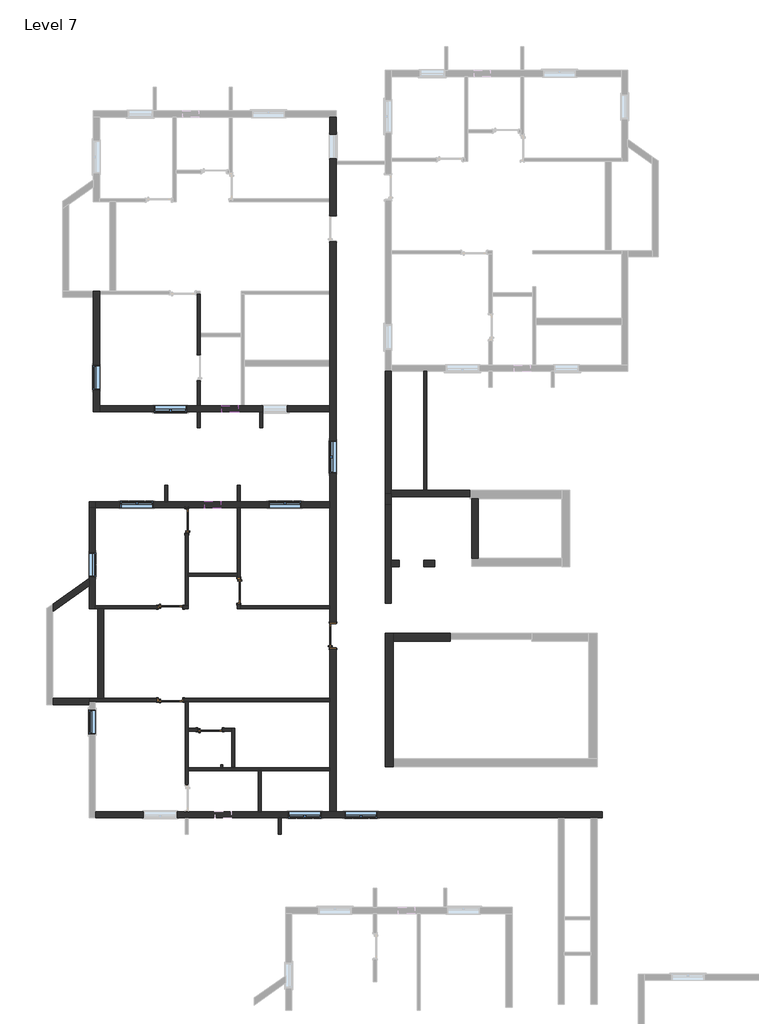
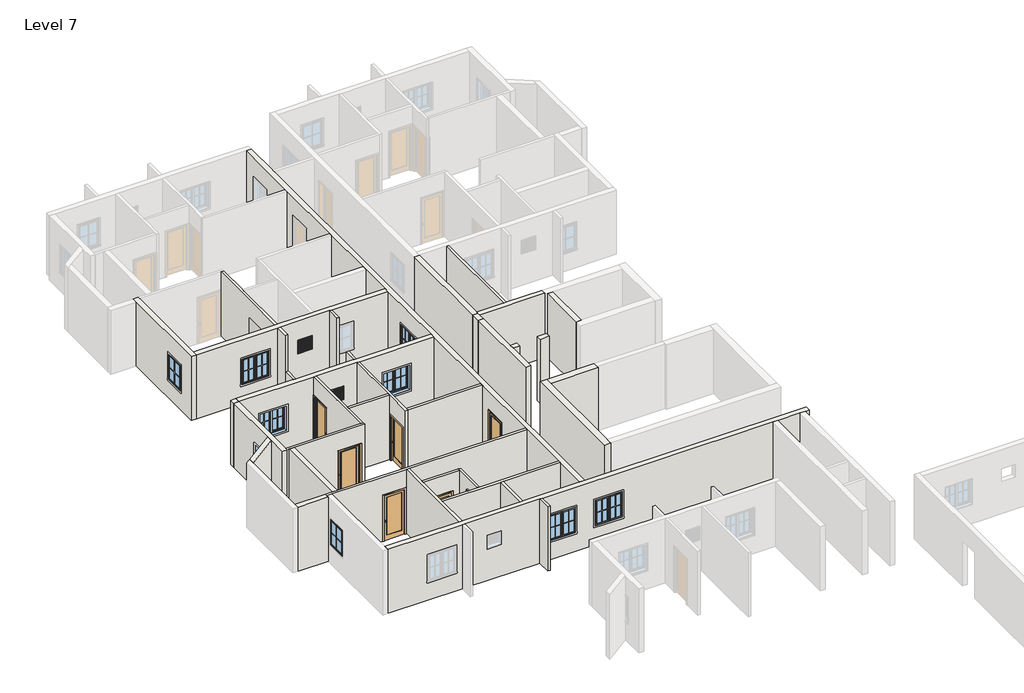
# One storey, part 4 of 7: 38 walls, 11 windows, 6 doors.
"""IFC4 building model written with IfcOpenShell, lengths in millimetres."""

from ifc_helpers import new_model, si_unit, frame, origin, place, context, project, spatial, polyline, outline, extrude, faceted_brep, transform, mapped, element, save
from components import door_a3feeac7, door_3c6ab76a, door_3b97b8e7, window_272f20d6, window_casement_double_4_x_4_af3140d2, window_f2d8fef0

model = new_model("IFC4")

# Units and contexts
model_context = context("Model", 3, world=origin())
ifc_project = project(units=[si_unit("LENGTHUNIT", "METRE", prefix="MILLI")], contexts=[model_context])

# Site, building, storey
site = spatial("IfcSite", under=ifc_project)
building = spatial("IfcBuilding", under=site)
storey = spatial("IfcBuildingStorey", under=building, Name="Level 7", Elevation=9601.2)

# Doors
placement = place(None, origin())
door_shape = door_a3feeac7(model_context)
element("IfcDoor", 1, ObjectType="Door-Interior-Single-1_Panel-Wood : 2'6\" x 7' door", at=placement, inside=storey, context=model_context, shape_type="MappedRepresentation", body=[
    mapped(door_shape, transform((-11252.4759469, 12427.2461172, 9601.2), x_axis=(0.0, 1.0, 0.0), y_axis=(-1.0, 0.0, 0.0), z_axis=(0.0, 0.0, 1.0))),
])
element("IfcDoor", 2, ObjectType="Door-Interior-Single-1_Panel-Wood : 2'6\" x 7' door", at=placement, inside=storey, context=model_context, shape_type="MappedRepresentation", body=[
    mapped(door_shape, transform((-10385.7009469, 4632.6211172, 9601.2), x_axis=(1.0, 0.0, 0.0), y_axis=(0.0, 1.0, 0.0), z_axis=(0.0, 0.0, 1.0))),
])
door_2_shape = door_3c6ab76a(model_context)
element("IfcDoor", 3, ObjectType="Door-Interior-Single-1_Panel-Wood : 36\" x 84\"", at=placement, inside=storey, context=model_context, shape_type="MappedRepresentation", body=[
    mapped(door_2_shape, transform((-9309.3759469, 9817.3961172, 9601.2), x_axis=(0.0, -1.0, 0.0), y_axis=(1.0, 0.0, 0.0), z_axis=(0.0, 0.0, 1.0))),
])
element("IfcDoor", 4, ObjectType="Door-Interior-Single-1_Panel-Wood : 36\" x 84\"", at=placement, inside=storey, context=model_context, shape_type="MappedRepresentation", body=[
    mapped(door_2_shape, transform((-11865.2509469, 9210.9711172, 9601.2), x_axis=(1.0, 0.0, 0.0), y_axis=(0.0, 1.0, 0.0), z_axis=(0.0, 0.0, 1.0))),
])
door_3_shape = door_3b97b8e7(model_context)
element("IfcDoor", 5, ObjectType="Door-Interior-Single-1_Panel-Wood : 36\" x 84\"", at=placement, inside=storey, context=model_context, shape_type="MappedRepresentation", body=[
    mapped(door_3_shape, transform((-5791.4759469, 8140.9961172, 9601.2), x_axis=(0.0, 1.0, 0.0), y_axis=(-1.0, 0.0, 0.0), z_axis=(0.0, 0.0, 1.0))),
])
element("IfcDoor", 6, ObjectType="Door-Interior-Single-1_Panel-Wood : 36\" x 84\"", at=placement, inside=storey, context=model_context, shape_type="MappedRepresentation", body=[
    mapped(door_shape, transform((-11865.2509469, 5737.5211172, 9601.2), x_axis=(1.0, 0.0, 0.0), y_axis=(0.0, 1.0, 0.0), z_axis=(0.0, 0.0, 1.0))),
])

# Walls
element("IfcWall", 7, ObjectType="1' feet", at=placement, inside=storey, context=model_context, shape_type="Brep", body=[
    faceted_brep([(-3540.4009469, 3245.1461172, 9601.2), (-3540.4009469, 3549.9461172, 9601.2), (-3540.4009469, 7931.4461172, 9601.2), (-3540.4009469, 8236.2461172, 9601.2), (-3540.4009469, 8236.2461172, 12649.2), (-3540.4009469, 7931.4461172, 12649.2), (-3540.4009469, 3549.9461172, 12649.2), (-3540.4009469, 3245.1461172, 12649.2), (-3845.2009469, 3245.1461172, 9601.2), (-3845.2009469, 3245.1461172, 12649.2), (-3845.2009469, 8236.2461172, 12649.2), (-3845.2009469, 8236.2461172, 9601.2)], [[[0, 1, 2, 3, 4, 5, 6, 7]], [[8, 9, 10, 11]], [[3, 2, 1, 0, 8, 11]], [[7, 6, 5, 4, 10, 9]], [[4, 3, 11, 10]], [[0, 7, 9, 8]]]),
])
element("IfcWall", 8, ObjectType="1' feet", at=placement, inside=storey, context=model_context, shape_type="Brep", body=[
    faceted_brep([(-3540.4009469, 7931.4461172, 9601.2), (-1406.8009469, 7931.4461172, 9601.2), (-1406.8009469, 7931.4461172, 12649.2), (-3540.4009469, 7931.4461172, 12649.2), (-3540.4009469, 8236.2461172, 9601.2), (-3540.4009469, 8236.2461172, 12649.2), (-1406.8009469, 8236.2461172, 12649.2), (-1406.8009469, 8236.2461172, 9601.2), (-1406.8009469, 8007.6461172, 9601.2), (-1406.8009469, 8007.6461172, 12649.2)], [[[0, 1, 2, 3]], [[4, 5, 6, 7]], [[1, 0, 4, 7, 8]], [[2, 1, 8, 7, 6, 9]], [[3, 2, 9, 6, 5]], [[0, 3, 5, 4]]]),
])
element("IfcWall", 9, ObjectType="4.5\" wall", at=placement, inside=storey, context=model_context, shape_type="Brep", body=[
    faceted_brep([(-10741.3009469, 20898.1461172, 12649.2), (-10741.3009469, 19437.6461172, 12649.2), (-10741.3009469, 19323.3461172, 12649.2), (-10741.3009469, 16732.5461172, 12649.2), (-10741.3009469, 16732.5461172, 9601.2), (-10741.3009469, 17678.6961172, 9601.2), (-10741.3009469, 17678.6961172, 11760.2), (-10741.3009469, 18643.8961172, 11760.2), (-10741.3009469, 18643.8961172, 9601.2), (-10741.3009469, 19323.3461172, 9601.2), (-10741.3009469, 19437.6461172, 9601.2), (-10741.3009469, 20898.1461172, 9601.2), (-10855.6009469, 16732.5461172, 12649.2), (-10855.6009469, 20898.1461172, 12649.2), (-10855.6009469, 20898.1461172, 9601.2), (-10855.6009469, 18643.8961172, 9601.2), (-10855.6009469, 18643.8961172, 11760.2), (-10855.6009469, 17678.6961172, 11760.2), (-10855.6009469, 17678.6961172, 9601.2), (-10855.6009469, 16732.5461172, 9601.2)], [[[0, 1, 2, 3, 4, 5, 6, 7, 8, 9, 10, 11]], [[12, 13, 14, 15, 16, 17, 18, 19]], [[4, 19, 18, 5]], [[14, 11, 10, 9, 8, 15]], [[3, 2, 1, 0, 13, 12]], [[4, 3, 12, 19]], [[0, 11, 14, 13]], [[7, 16, 15, 8]], [[16, 7, 6, 17]], [[17, 6, 5, 18]]]),
])
element("IfcWall", 10, ObjectType="4.5\" wall", at=placement, inside=storey, context=model_context, shape_type="Brep", body=[
    faceted_brep([(-9369.7009469, 9150.6461172, 12649.2), (-9369.7009469, 10369.8461172, 12649.2), (-9369.7009469, 10484.1461172, 12649.2), (-9369.7009469, 12922.5461172, 12649.2), (-9369.7009469, 12922.5461172, 9601.2), (-9369.7009469, 10484.1461172, 9601.2), (-9369.7009469, 10369.8461172, 9601.2), (-9369.7009469, 10299.9961172, 9601.2), (-9369.7009469, 10299.9961172, 11760.2), (-9369.7009469, 9334.7961172, 11760.2), (-9369.7009469, 9334.7961172, 9601.2), (-9369.7009469, 9150.6461172, 9601.2), (-9255.4009469, 12922.5461172, 12649.2), (-9255.4009469, 9264.9461172, 12649.2), (-9255.4009469, 9150.6461172, 12649.2), (-9255.4009469, 9150.6461172, 9601.2), (-9255.4009469, 9264.9461172, 9601.2), (-9255.4009469, 9334.7961172, 9601.2), (-9255.4009469, 9334.7961172, 11760.2), (-9255.4009469, 10299.9961172, 11760.2), (-9255.4009469, 10299.9961172, 9601.2), (-9255.4009469, 12922.5461172, 9601.2)], [[[0, 1, 2, 3, 4, 5, 6, 7, 8, 9, 10, 11]], [[12, 13, 14, 15, 16, 17, 18, 19, 20, 21]], [[4, 21, 20, 7, 6, 5]], [[15, 11, 10, 17, 16]], [[3, 2, 1, 0, 14, 13, 12]], [[4, 3, 12, 21]], [[0, 11, 15, 14]], [[9, 18, 17, 10]], [[18, 9, 8, 19]], [[19, 8, 7, 20]]]),
])
element("IfcWall", 11, ObjectType="4.5\" wall", at=placement, inside=storey, context=model_context, shape_type="SweptSolid", body=[
    extrude(outline(polyline([(-11198.5009469, 10484.1461172), (-9369.7009469, 10484.1461172), (-9369.7009469, 10369.8461172), (-11198.5009469, 10369.8461172), (-11198.5009469, 10484.1461172)])), frame((0.0, 0.0, 9601.2), z_axis=(0.0, 0.0, 1.0), x_axis=(1.0, 0.0, 0.0)), (0.0, 0.0, 1.0), 3048.0),
])
element("IfcWall", 12, ObjectType="4.5\" wall", at=placement, inside=storey, context=model_context, shape_type="Brep", body=[
    faceted_brep([(-11312.8009469, 9264.9461172, 12649.2), (-11312.8009469, 12922.5461172, 12649.2), (-11312.8009469, 12922.5461172, 9601.2), (-11312.8009469, 12909.8461172, 9601.2), (-11312.8009469, 12909.8461172, 11760.2), (-11312.8009469, 11944.6461172, 11760.2), (-11312.8009469, 11944.6461172, 9601.2), (-11312.8009469, 9264.9461172, 9601.2), (-11198.5009469, 12922.5461172, 12649.2), (-11198.5009469, 10484.1461172, 12649.2), (-11198.5009469, 10369.8461172, 12649.2), (-11198.5009469, 9264.9461172, 12649.2), (-11198.5009469, 9264.9461172, 9601.2), (-11198.5009469, 10369.8461172, 9601.2), (-11198.5009469, 10484.1461172, 9601.2), (-11198.5009469, 11944.6461172, 9601.2), (-11198.5009469, 11944.6461172, 11760.2), (-11198.5009469, 12909.8461172, 11760.2), (-11198.5009469, 12909.8461172, 9601.2), (-11198.5009469, 12922.5461172, 9601.2)], [[[0, 1, 2, 3, 4, 5, 6, 7]], [[8, 9, 10, 11, 12, 13, 14, 15, 16, 17, 18, 19]], [[12, 7, 6, 15, 14, 13]], [[2, 19, 18, 3]], [[1, 0, 11, 10, 9, 8]], [[0, 7, 12, 11]], [[2, 1, 8, 19]], [[17, 4, 3, 18]], [[4, 17, 16, 5]], [[5, 16, 15, 6]]]),
])
element("IfcWall", 13, ObjectType="4.5\" wall", at=placement, inside=storey, context=model_context, shape_type="Brep", body=[
    faceted_brep([(-14665.6009469, 9264.9461172, 12649.2), (-11312.8009469, 9264.9461172, 12649.2), (-11198.5009469, 9264.9461172, 12649.2), (-11198.5009469, 9264.9461172, 9601.2), (-11312.8009469, 9264.9461172, 9601.2), (-11382.6509469, 9264.9461172, 9601.2), (-11382.6509469, 9264.9461172, 11760.2), (-12347.8509469, 9264.9461172, 11760.2), (-12347.8509469, 9264.9461172, 9601.2), (-14665.6009469, 9264.9461172, 9601.2), (-11198.5009469, 9150.6461172, 12649.2), (-14360.8009469, 9150.6461172, 12649.2), (-14589.4009469, 9150.6461172, 12649.2), (-14665.6009469, 9150.6461172, 12649.2), (-14665.6009469, 9150.6461172, 9601.2), (-14589.4009469, 9150.6461172, 9601.2), (-14360.8009469, 9150.6461172, 9601.2), (-12347.8509469, 9150.6461172, 9601.2), (-12347.8509469, 9150.6461172, 11760.2), (-11382.6509469, 9150.6461172, 11760.2), (-11382.6509469, 9150.6461172, 9601.2), (-11198.5009469, 9150.6461172, 9601.2)], [[[0, 1, 2, 3, 4, 5, 6, 7, 8, 9]], [[10, 11, 12, 13, 14, 15, 16, 17, 18, 19, 20, 21]], [[3, 21, 20, 5, 4]], [[14, 9, 8, 17, 16, 15]], [[2, 1, 0, 13, 12, 11, 10]], [[3, 2, 10, 21]], [[0, 9, 14, 13]], [[19, 6, 5, 20]], [[6, 19, 18, 7]], [[7, 18, 17, 8]]]),
])
element("IfcWall", 14, ObjectType="4.5\" wall", at=placement, inside=storey, context=model_context, shape_type="SweptSolid", body=[
    extrude(outline(polyline([(-9255.4009469, 9264.9461172), (-5902.6009469, 9264.9461172), (-5902.6009469, 9150.6461172), (-9255.4009469, 9150.6461172), (-9255.4009469, 9264.9461172)])), frame((0.0, 0.0, 9601.2), z_axis=(0.0, 0.0, 1.0), x_axis=(1.0, 0.0, 0.0)), (0.0, 0.0, 1.0), 3048.0),
])
element("IfcWall", 15, ObjectType="4.5\" wall", at=placement, inside=storey, context=model_context, shape_type="Brep", body=[
    faceted_brep([(-5902.6009469, 5683.5461172, 12649.2), (-11198.5009469, 5683.5461172, 12649.2), (-11312.8009469, 5683.5461172, 12649.2), (-14665.6009469, 5683.5461172, 12649.2), (-14894.2009469, 5683.5461172, 12649.2), (-14894.2009469, 5683.5461172, 9601.2), (-14665.6009469, 5683.5461172, 9601.2), (-12347.8509469, 5683.5461172, 9601.2), (-12347.8509469, 5683.5461172, 11760.2), (-11382.6509469, 5683.5461172, 11760.2), (-11382.6509469, 5683.5461172, 9601.2), (-11312.8009469, 5683.5461172, 9601.2), (-11198.5009469, 5683.5461172, 9601.2), (-5902.6009469, 5683.5461172, 9601.2), (-14894.2009469, 5797.8461172, 12649.2), (-14589.4009469, 5797.8461172, 12649.2), (-14360.8009469, 5797.8461172, 12649.2), (-5902.6009469, 5797.8461172, 12649.2), (-5902.6009469, 5797.8461172, 9601.2), (-11382.6509469, 5797.8461172, 9601.2), (-11382.6509469, 5797.8461172, 11760.2), (-12347.8509469, 5797.8461172, 11760.2), (-12347.8509469, 5797.8461172, 9601.2), (-14360.8009469, 5797.8461172, 9601.2), (-14589.4009469, 5797.8461172, 9601.2), (-14894.2009469, 5797.8461172, 9601.2)], [[[0, 1, 2, 3, 4, 5, 6, 7, 8, 9, 10, 11, 12, 13]], [[14, 15, 16, 17, 18, 19, 20, 21, 22, 23, 24, 25]], [[18, 13, 12, 11, 10, 19]], [[5, 25, 24, 23, 22, 7, 6]], [[4, 3, 2, 1, 0, 17, 16, 15, 14]], [[0, 13, 18, 17]], [[5, 4, 14, 25]], [[9, 20, 19, 10]], [[20, 9, 8, 21]], [[21, 8, 7, 22]]]),
])
element("IfcWall", 16, ObjectType="4.5\" wall", at=placement, inside=storey, context=model_context, shape_type="Brep", body=[
    faceted_brep([(-11198.5009469, 5683.5461172, 12649.2), (-11198.5009469, 4692.9461172, 12649.2), (-11198.5009469, 4578.6461172, 12649.2), (-11198.5009469, 3207.0461172, 12649.2), (-11198.5009469, 3092.7461172, 12649.2), (-11198.5009469, 1568.7461172, 12649.2), (-11198.5009469, 1568.7461172, 9601.2), (-11198.5009469, 1581.4461172, 9601.2), (-11198.5009469, 1581.4461172, 11760.2), (-11198.5009469, 2546.6461172, 11760.2), (-11198.5009469, 2546.6461172, 9601.2), (-11198.5009469, 3092.7461172, 9601.2), (-11198.5009469, 3207.0461172, 9601.2), (-11198.5009469, 4578.6461172, 9601.2), (-11198.5009469, 4692.9461172, 9601.2), (-11198.5009469, 5683.5461172, 9601.2), (-11312.8009469, 1568.7461172, 12649.2), (-11312.8009469, 5683.5461172, 12649.2), (-11312.8009469, 5683.5461172, 9601.2), (-11312.8009469, 2546.6461172, 9601.2), (-11312.8009469, 2546.6461172, 11760.2), (-11312.8009469, 1581.4461172, 11760.2), (-11312.8009469, 1581.4461172, 9601.2), (-11312.8009469, 1568.7461172, 9601.2)], [[[0, 1, 2, 3, 4, 5, 6, 7, 8, 9, 10, 11, 12, 13, 14, 15]], [[16, 17, 18, 19, 20, 21, 22, 23]], [[18, 15, 14, 13, 12, 11, 10, 19]], [[6, 23, 22, 7]], [[5, 4, 3, 2, 1, 0, 17, 16]], [[0, 15, 18, 17]], [[6, 5, 16, 23]], [[21, 8, 7, 22]], [[8, 21, 20, 9]], [[9, 20, 19, 10]]]),
])
element("IfcWall", 17, ObjectType="4.5\" wall", at=placement, inside=storey, context=model_context, shape_type="SweptSolid", body=[
    extrude(outline(polyline([(-9985.226836, 3326.5226372), (-9915.376836, 3326.5226372), (-9915.376836, 3212.2226372), (-9985.226836, 3212.2226372), (-9985.226836, 3326.5226372)])), frame((0.0, 0.0, 9601.2), z_axis=(0.0, 0.0, 1.0), x_axis=(1.0, 0.0, 0.0)), (0.0, 0.0, 1.0), 3048.0),
])
element("IfcWall", 18, ObjectType="4.5\" wall", at=placement, inside=storey, context=model_context, shape_type="Brep", body=[
    faceted_brep([(-5902.6009469, 3207.0461172, 9601.2), (-11198.5009469, 3207.0461172, 9601.2), (-11198.5009469, 3207.0461172, 12649.2), (-5902.6009469, 3207.0461172, 12649.2), (-5902.6009469, 3092.7461172, 9601.2), (-5902.6009469, 3092.7461172, 12649.2), (-8468.0009469, 3092.7461172, 12649.2), (-8582.3009469, 3092.7461172, 12649.2), (-11198.5009469, 3092.7461172, 12649.2), (-11198.5009469, 3092.7461172, 9601.2), (-8582.3009469, 3092.7461172, 9601.2), (-8468.0009469, 3092.7461172, 9601.2)], [[[0, 1, 2, 3]], [[4, 5, 6, 7, 8, 9, 10, 11]], [[1, 0, 4, 11, 10, 9]], [[3, 2, 8, 7, 6, 5]], [[2, 1, 9, 8]], [[0, 3, 5, 4]]]),
])
element("IfcWall", 19, ObjectType="4.5\" wall", at=placement, inside=storey, context=model_context, shape_type="SweptSolid", body=[
    extrude(outline(polyline([(-8582.3009469, 1568.7461172), (-8582.3009469, 3092.7461172), (-8468.0009469, 3092.7461172), (-8468.0009469, 1568.7461172), (-8582.3009469, 1568.7461172)])), frame((0.0, 0.0, 9601.2), z_axis=(0.0, 0.0, 1.0), x_axis=(1.0, 0.0, 0.0)), (0.0, 0.0, 1.0), 3048.0),
])
element("IfcWall", 20, ObjectType="4.5\" wall", at=placement, inside=storey, context=model_context, shape_type="Brep", body=[
    faceted_brep([(-9572.9009469, 4692.9461172, 9601.2), (-9572.9009469, 4578.6461172, 9601.2), (-9572.9009469, 3245.1461172, 9601.2), (-9572.9009469, 3245.1461172, 12649.2), (-9572.9009469, 4578.6461172, 12649.2), (-9572.9009469, 4692.9461172, 12649.2), (-9458.6009469, 4692.9461172, 9601.2), (-9458.6009469, 4692.9461172, 12649.2), (-9458.6009469, 3245.1461172, 12649.2), (-9458.6009469, 3245.1461172, 9601.2)], [[[0, 1, 2, 3, 4, 5]], [[6, 7, 8, 9]], [[2, 1, 0, 6, 9]], [[3, 2, 9, 8]], [[5, 4, 3, 8, 7]], [[0, 5, 7, 6]]]),
])
element("IfcWall", 21, ObjectType="4.5\" wall", at=placement, inside=storey, context=model_context, shape_type="SweptSolid", body=[
    extrude(outline(polyline([(12649.2, -9572.9009469), (12649.2, -11198.5009469), (9601.2, -11198.5009469), (9601.2, -10868.3009469), (11760.2, -10868.3009469), (11760.2, -9903.1009469), (9601.2, -9903.1009469), (9601.2, -9572.9009469), (12649.2, -9572.9009469)])), frame((0.0, 4578.6461172, 0.0), z_axis=(0.0, 1.0, 0.0), x_axis=(0.0, 0.0, 1.0)), (0.0, 0.0, 1.0), 114.3),
])
element("IfcWall", 22, ObjectType="4.5\" wall", at=placement, inside=storey, context=model_context, shape_type="SweptSolid", body=[
    extrude(outline(polyline([(-7841.0333092, 730.5461172), (-7841.0333092, 1340.1461172), (-7726.7333092, 1340.1461172), (-7726.7333092, 730.5461172), (-7841.0333092, 730.5461172)])), frame((0.0, 0.0, 9601.2), z_axis=(0.0, 0.0, 1.0), x_axis=(1.0, 0.0, 0.0)), (0.0, 0.0, 1.0), 3048.0),
])
element("IfcWall", 23, ObjectType="4.5\" wall", at=placement, inside=storey, context=model_context, shape_type="SweptSolid", body=[
    extrude(outline(polyline([(-10855.6009469, 15918.3895495), (-10855.6009469, 16503.9461172), (-10741.3009469, 16503.9461172), (-10741.3009469, 15918.3895495), (-10855.6009469, 15918.3895495)])), frame((0.0, 0.0, 9601.2), z_axis=(0.0, 0.0, 1.0), x_axis=(1.0, 0.0, 0.0)), (0.0, 0.0, 1.0), 3048.0),
])
element("IfcWall", 24, ObjectType="4.5\" wall", at=placement, inside=storey, context=model_context, shape_type="Brep", body=[
    faceted_brep([(-8531.5009469, 16503.9461172, 9601.2), (-8531.5009469, 15918.3895495, 9601.2), (-8531.5009469, 15918.3895495, 12649.2), (-8531.5009469, 16503.9461172, 12649.2), (-8417.2009469, 16503.9461172, 9601.2), (-8417.2009469, 16503.9461172, 10515.6), (-8417.2009469, 16503.9461172, 11734.8), (-8417.2009469, 16503.9461172, 12649.2), (-8417.2009469, 15918.3895495, 12649.2), (-8417.2009469, 15918.3895495, 9601.2)], [[[0, 1, 2, 3]], [[4, 5, 6, 7, 8, 9]], [[1, 0, 4, 9]], [[2, 1, 9, 8]], [[3, 2, 8, 7]], [[0, 3, 7, 6, 5, 4]]]),
])
element("IfcWall", 25, ObjectType="4.5\" wall", at=placement, inside=storey, context=model_context, shape_type="SweptSolid", body=[
    extrude(outline(polyline([(-12085.9698258, 13151.1461172), (-12085.9698258, 13760.7461172), (-11971.6698258, 13760.7461172), (-11971.6698258, 13151.1461172), (-12085.9698258, 13151.1461172)])), frame((0.0, 0.0, 9601.2), z_axis=(0.0, 0.0, 1.0), x_axis=(1.0, 0.0, 0.0)), (0.0, 0.0, 1.0), 3048.0),
])
element("IfcWall", 26, ObjectType="4.5\" wall", at=placement, inside=storey, context=model_context, shape_type="SweptSolid", body=[
    extrude(outline(polyline([(-9255.4009469, 13760.7461172), (-9255.4009469, 13151.1461172), (-9369.7009469, 13151.1461172), (-9369.7009469, 13760.7461172), (-9255.4009469, 13760.7461172)])), frame((0.0, 0.0, 9601.2), z_axis=(0.0, 0.0, 1.0), x_axis=(1.0, 0.0, 0.0)), (0.0, 0.0, 1.0), 3048.0),
])
element("IfcWall", 27, ObjectType="4.5\" wall", at=placement, inside=storey, context=model_context, shape_type="SweptSolid", body=[
    extrude(outline(polyline([(-2402.381873, 13571.4182723), (-2402.381873, 18017.4255084), (-2288.081873, 18017.4255084), (-2288.081873, 13571.4182723), (-2402.381873, 13571.4182723)])), frame((0.0, 0.0, 9601.2), z_axis=(0.0, 0.0, 1.0), x_axis=(1.0, 0.0, 0.0)), (0.0, 0.0, 1.0), 3048.0),
])
element("IfcWall", 28, ObjectType="9\"", at=placement, inside=storey, context=model_context, shape_type="Brep", body=[
    faceted_brep([(-14513.2009469, 16503.9461172, 9601.2), (-14513.2009469, 16732.5461172, 9601.2), (-14513.2009469, 20898.1461172, 9601.2), (-14513.2009469, 21012.4461172, 9601.2), (-14513.2009469, 21012.4461172, 12649.2), (-14513.2009469, 20898.1461172, 12649.2), (-14513.2009469, 16732.5461172, 12649.2), (-14513.2009469, 16503.9461172, 12649.2), (-14513.2009469, 18243.8461172, 11734.8), (-14513.2009469, 18243.8461172, 10515.6), (-14513.2009469, 17329.4461172, 10515.6), (-14513.2009469, 17329.4461172, 11734.8), (-14741.8009469, 16503.9461172, 9601.2), (-14741.8009469, 16503.9461172, 12649.2), (-14741.8009469, 20783.8461172, 12649.2), (-14741.8009469, 21012.4461172, 12649.2), (-14741.8009469, 21012.4461172, 9601.2), (-14741.8009469, 20783.8461172, 9601.2), (-14741.8009469, 18243.8461172, 11734.8), (-14741.8009469, 17329.4461172, 11734.8), (-14741.8009469, 17329.4461172, 10515.6), (-14741.8009469, 18243.8461172, 10515.6)], [[[0, 1, 2, 3, 4, 5, 6, 7], [8, 9, 10, 11]], [[12, 13, 14, 15, 16, 17], [18, 19, 20, 21]], [[3, 2, 1, 0, 12, 17, 16]], [[7, 6, 5, 4, 15, 14, 13]], [[4, 3, 16, 15]], [[0, 7, 13, 12]], [[9, 8, 18, 21]], [[10, 9, 21, 20]], [[11, 10, 20, 19]], [[8, 11, 19, 18]]]),
])
element("IfcWall", 29, ObjectType="9\"", at=placement, inside=storey, context=model_context, shape_type="Brep", body=[
    faceted_brep([(-5902.6009469, 1568.7461172, 12649.2), (-5902.6009469, 3092.7461172, 12649.2), (-5902.6009469, 3207.0461172, 12649.2), (-5902.6009469, 5683.5461172, 12649.2), (-5902.6009469, 5797.8461172, 12649.2), (-5902.6009469, 9150.6461172, 12649.2), (-5902.6009469, 9264.9461172, 12649.2), (-5902.6009469, 12922.5461172, 12649.2), (-5902.6009469, 13151.1461172, 12649.2), (-5902.6009469, 16503.9461172, 12649.2), (-5902.6009469, 16732.5461172, 12649.2), (-5902.6009469, 18205.7461172, 12649.2), (-5902.6009469, 18434.3461172, 12649.2), (-5902.6009469, 20898.1461172, 12649.2), (-5902.6009469, 21012.4461172, 12649.2), (-5902.6009469, 24365.2461172, 12649.2), (-5902.6009469, 24479.5461172, 12649.2), (-5902.6009469, 27527.5461172, 12649.2), (-5902.6009469, 27527.5461172, 9601.2), (-5902.6009469, 24479.5461172, 9601.2), (-5902.6009469, 24365.2461172, 9601.2), (-5902.6009469, 23838.1961172, 9601.2), (-5902.6009469, 23838.1961172, 11760.2), (-5902.6009469, 22872.9961172, 11760.2), (-5902.6009469, 22872.9961172, 9601.2), (-5902.6009469, 21012.4461172, 9601.2), (-5902.6009469, 20898.1461172, 9601.2), (-5902.6009469, 18434.3461172, 9601.2), (-5902.6009469, 18205.7461172, 9601.2), (-5902.6009469, 16732.5461172, 9601.2), (-5902.6009469, 16503.9461172, 9601.2), (-5902.6009469, 13151.1461172, 9601.2), (-5902.6009469, 12922.5461172, 9601.2), (-5902.6009469, 9264.9461172, 9601.2), (-5902.6009469, 9150.6461172, 9601.2), (-5902.6009469, 8623.5961172, 9601.2), (-5902.6009469, 8623.5961172, 11760.2), (-5902.6009469, 7658.3961172, 11760.2), (-5902.6009469, 7658.3961172, 9601.2), (-5902.6009469, 5797.8461172, 9601.2), (-5902.6009469, 5683.5461172, 9601.2), (-5902.6009469, 3207.0461172, 9601.2), (-5902.6009469, 3092.7461172, 9601.2), (-5902.6009469, 1568.7461172, 9601.2), (-5902.6009469, 25973.9755084, 11734.8), (-5902.6009469, 25973.9755084, 10515.6), (-5902.6009469, 26888.3755084, 10515.6), (-5902.6009469, 26888.3755084, 11734.8), (-5902.6009469, 15437.1461172, 11734.8), (-5902.6009469, 14217.9461172, 11734.8), (-5902.6009469, 14217.9461172, 10515.6), (-5902.6009469, 15437.1461172, 10515.6), (-5674.0009469, 27527.5461172, 12649.2), (-5674.0009469, 25878.7255084, 12649.2), (-5674.0009469, 25764.4255084, 12649.2), (-5674.0009469, 1568.7461172, 12649.2), (-5674.0009469, 1568.7461172, 9601.2), (-5674.0009469, 7658.3961172, 9601.2), (-5674.0009469, 7658.3961172, 11760.2), (-5674.0009469, 8623.5961172, 11760.2), (-5674.0009469, 8623.5961172, 9601.2), (-5674.0009469, 22872.9961172, 9601.2), (-5674.0009469, 22872.9961172, 11760.2), (-5674.0009469, 23838.1961172, 11760.2), (-5674.0009469, 23838.1961172, 9601.2), (-5674.0009469, 25764.4255084, 9601.2), (-5674.0009469, 25878.7255084, 9601.2), (-5674.0009469, 27527.5461172, 9601.2), (-5674.0009469, 27527.5461172, 9753.6), (-5674.0009469, 25973.9755084, 11734.8), (-5674.0009469, 26888.3755084, 11734.8), (-5674.0009469, 26888.3755084, 10515.6), (-5674.0009469, 25973.9755084, 10515.6), (-5674.0009469, 15437.1461172, 11734.8), (-5674.0009469, 15437.1461172, 10515.6), (-5674.0009469, 14217.9461172, 10515.6), (-5674.0009469, 14217.9461172, 11734.8)], [[[0, 1, 2, 3, 4, 5, 6, 7, 8, 9, 10, 11, 12, 13, 14, 15, 16, 17, 18, 19, 20, 21, 22, 23, 24, 25, 26, 27, 28, 29, 30, 31, 32, 33, 34, 35, 36, 37, 38, 39, 40, 41, 42, 43], [44, 45, 46, 47], [48, 49, 50, 51]], [[52, 53, 54, 55, 56, 57, 58, 59, 60, 61, 62, 63, 64, 65, 66, 67, 68], [69, 70, 71, 72], [73, 74, 75, 76]], [[18, 67, 66, 65, 64, 21, 20, 19]], [[56, 43, 42, 41, 40, 39, 38, 57]], [[24, 61, 60, 35, 34, 33, 32, 31, 30, 29, 28, 27, 26, 25]], [[17, 16, 15, 14, 13, 12, 11, 10, 9, 8, 7, 6, 5, 4, 3, 2, 1, 0, 55, 54, 53, 52]], [[18, 17, 52, 68, 67]], [[0, 43, 56, 55]], [[63, 22, 21, 64]], [[22, 63, 62, 23]], [[23, 62, 61, 24]], [[59, 36, 35, 60]], [[36, 59, 58, 37]], [[37, 58, 57, 38]], [[45, 44, 69, 72]], [[46, 45, 72, 71]], [[47, 46, 71, 70]], [[44, 47, 70, 69]], [[74, 73, 48, 51]], [[75, 74, 51, 50]], [[76, 75, 50, 49]], [[73, 76, 49, 48]]]),
])
element("IfcWall", 30, ObjectType="9\"", at=placement, inside=storey, context=model_context, shape_type="Brep", body=[
    faceted_brep([(-14513.2009469, 16503.9461172, 9601.2), (-10855.6009469, 16503.9461172, 9601.2), (-10741.3009469, 16503.9461172, 9601.2), (-8531.5009469, 16503.9461172, 9601.2), (-8417.2009469, 16503.9461172, 9601.2), (-5902.6009469, 16503.9461172, 9601.2), (-5902.6009469, 16503.9461172, 12649.2), (-8417.2009469, 16503.9461172, 12649.2), (-8531.5009469, 16503.9461172, 12649.2), (-10741.3009469, 16503.9461172, 12649.2), (-10855.6009469, 16503.9461172, 12649.2), (-14513.2009469, 16503.9461172, 12649.2), (-9337.9509469, 16503.9461172, 11734.8), (-9337.9509469, 16503.9461172, 11125.2), (-9947.5509469, 16503.9461172, 11125.2), (-9947.5509469, 16503.9461172, 11734.8), (-8417.2009469, 16503.9461172, 11734.8), (-7502.8009469, 16503.9461172, 11734.8), (-7502.8009469, 16503.9461172, 10515.6), (-8417.2009469, 16503.9461172, 10515.6), (-12474.8509469, 16503.9461172, 11734.8), (-11255.6509469, 16503.9461172, 11734.8), (-11255.6509469, 16503.9461172, 10515.6), (-12474.8509469, 16503.9461172, 10515.6), (-14513.2009469, 16732.5461172, 9601.2), (-14513.2009469, 16732.5461172, 12649.2), (-10855.6009469, 16732.5461172, 12649.2), (-10741.3009469, 16732.5461172, 12649.2), (-9217.3009469, 16732.5461172, 12649.2), (-9103.0009469, 16732.5461172, 12649.2), (-5902.6009469, 16732.5461172, 12649.2), (-5902.6009469, 16732.5461172, 9601.2), (-9103.0009469, 16732.5461172, 9601.2), (-9217.3009469, 16732.5461172, 9601.2), (-10741.3009469, 16732.5461172, 9601.2), (-10855.6009469, 16732.5461172, 9601.2), (-9337.9509469, 16732.5461172, 11734.8), (-9947.5509469, 16732.5461172, 11734.8), (-9947.5509469, 16732.5461172, 11125.2), (-9337.9509469, 16732.5461172, 11125.2), (-8417.2009469, 16732.5461172, 11734.8), (-8417.2009469, 16732.5461172, 10515.6), (-7502.8009469, 16732.5461172, 10515.6), (-7502.8009469, 16732.5461172, 11734.8), (-12474.8509469, 16732.5461172, 11734.8), (-12474.8509469, 16732.5461172, 10515.6), (-11255.6509469, 16732.5461172, 10515.6), (-11255.6509469, 16732.5461172, 11734.8)], [[[0, 1, 2, 3, 4, 5, 6, 7, 8, 9, 10, 11], [12, 13, 14, 15], [16, 17, 18, 19], [20, 21, 22, 23]], [[24, 25, 26, 27, 28, 29, 30, 31, 32, 33, 34, 35], [36, 37, 38, 39], [40, 41, 42, 43], [44, 45, 46, 47]], [[5, 4, 3, 2, 1, 0, 24, 35, 34, 33, 32, 31]], [[11, 10, 9, 8, 7, 6, 30, 29, 28, 27, 26, 25]], [[6, 5, 31, 30]], [[0, 11, 25, 24]], [[13, 12, 36, 39]], [[14, 13, 39, 38]], [[15, 14, 38, 37]], [[12, 15, 37, 36]], [[41, 40, 16, 19]], [[42, 41, 19, 18]], [[43, 42, 18, 17]], [[40, 43, 17, 16]], [[45, 44, 20, 23]], [[46, 45, 23, 22]], [[47, 46, 22, 21]], [[44, 47, 21, 20]]]),
])
element("IfcWall", 31, ObjectType="9\"", at=placement, inside=storey, context=model_context, shape_type="Brep", body=[
    faceted_brep([(-5902.6009469, 13151.1461172, 9601.2), (-9255.4009469, 13151.1461172, 9601.2), (-9369.7009469, 13151.1461172, 9601.2), (-11971.6698258, 13151.1461172, 9601.2), (-12085.9698258, 13151.1461172, 9601.2), (-14665.6009469, 13151.1461172, 9601.2), (-14665.6009469, 13151.1461172, 12649.2), (-12085.9698258, 13151.1461172, 12649.2), (-11971.6698258, 13151.1461172, 12649.2), (-9369.7009469, 13151.1461172, 12649.2), (-9255.4009469, 13151.1461172, 12649.2), (-5902.6009469, 13151.1461172, 12649.2), (-9979.3009469, 13151.1461172, 11734.8), (-10588.9009469, 13151.1461172, 11734.8), (-10588.9009469, 13151.1461172, 11125.2), (-9979.3009469, 13151.1461172, 11125.2), (-12511.4198258, 13151.1461172, 11734.8), (-13730.6198258, 13151.1461172, 11734.8), (-13730.6198258, 13151.1461172, 10515.6), (-12511.4198258, 13151.1461172, 10515.6), (-6975.7509469, 13151.1461172, 11734.8), (-8194.9509469, 13151.1461172, 11734.8), (-8194.9509469, 13151.1461172, 10515.6), (-6975.7509469, 13151.1461172, 10515.6), (-5902.6009469, 12922.5461172, 9601.2), (-5902.6009469, 12922.5461172, 12649.2), (-9255.4009469, 12922.5461172, 12649.2), (-9369.7009469, 12922.5461172, 12649.2), (-11198.5009469, 12922.5461172, 12649.2), (-11312.8009469, 12922.5461172, 12649.2), (-14665.6009469, 12922.5461172, 12649.2), (-14665.6009469, 12922.5461172, 9601.2), (-11312.8009469, 12922.5461172, 9601.2), (-11198.5009469, 12922.5461172, 9601.2), (-9369.7009469, 12922.5461172, 9601.2), (-9255.4009469, 12922.5461172, 9601.2), (-9979.3009469, 12922.5461172, 11734.8), (-9979.3009469, 12922.5461172, 11125.2), (-10588.9009469, 12922.5461172, 11125.2), (-10588.9009469, 12922.5461172, 11734.8), (-12511.4198258, 12922.5461172, 11734.8), (-12511.4198258, 12922.5461172, 10515.6), (-13730.6198258, 12922.5461172, 10515.6), (-13730.6198258, 12922.5461172, 11734.8), (-6975.7509469, 12922.5461172, 11734.8), (-6975.7509469, 12922.5461172, 10515.6), (-8194.9509469, 12922.5461172, 10515.6), (-8194.9509469, 12922.5461172, 11734.8)], [[[0, 1, 2, 3, 4, 5, 6, 7, 8, 9, 10, 11], [12, 13, 14, 15], [16, 17, 18, 19], [20, 21, 22, 23]], [[24, 25, 26, 27, 28, 29, 30, 31, 32, 33, 34, 35], [36, 37, 38, 39], [40, 41, 42, 43], [44, 45, 46, 47]], [[5, 4, 3, 2, 1, 0, 24, 35, 34, 33, 32, 31]], [[11, 10, 9, 8, 7, 6, 30, 29, 28, 27, 26, 25]], [[6, 5, 31, 30]], [[0, 11, 25, 24]], [[37, 36, 12, 15]], [[38, 37, 15, 14]], [[39, 38, 14, 13]], [[36, 39, 13, 12]], [[41, 40, 16, 19]], [[42, 41, 19, 18]], [[43, 42, 18, 17]], [[40, 43, 17, 16]], [[45, 44, 20, 23]], [[46, 45, 23, 22]], [[47, 46, 22, 21]], [[44, 47, 21, 20]]]),
])
element("IfcWall", 32, ObjectType="9\"", at=placement, inside=storey, context=model_context, shape_type="SweptSolid", body=[
    extrude(outline(polyline([(-14894.2009469, 12922.5461172), (-14894.2009469, 13151.1461172), (-14665.6009469, 13151.1461172), (-14665.6009469, 12922.5461172), (-14894.2009469, 12922.5461172)])), frame((0.0, 0.0, 9601.2), z_axis=(0.0, 0.0, 1.0), x_axis=(1.0, 0.0, 0.0)), (0.0, 0.0, 1.0), 3048.0),
])
element("IfcWall", 33, ObjectType="9\"", at=placement, inside=storey, context=model_context, shape_type="SweptSolid", body=[
    extrude(outline(polyline([(-14589.4009469, 5797.8461172), (-14589.4009469, 9150.6461172), (-14360.8009469, 9150.6461172), (-14360.8009469, 5797.8461172), (-14589.4009469, 5797.8461172)])), frame((0.0, 0.0, 9601.2), z_axis=(0.0, 0.0, 1.0), x_axis=(1.0, 0.0, 0.0)), (0.0, 0.0, 1.0), 3048.0),
])
element("IfcWall", 34, ObjectType="9\"", at=placement, inside=storey, context=model_context, shape_type="Brep", body=[
    faceted_brep([(-14665.6009469, 1340.1461172, 9601.2), (-11312.8009469, 1340.1461172, 9601.2), (-11198.5009469, 1340.1461172, 9601.2), (-7841.0333092, 1340.1461172, 9601.2), (-7726.7333092, 1340.1461172, 9601.2), (2631.7990531, 1340.1461172, 9601.2), (2860.3990531, 1340.1461172, 9601.2), (3850.9990531, 1340.1461172, 9601.2), (4079.5990531, 1340.1461172, 9601.2), (4270.0990531, 1340.1461172, 9601.2), (4270.0990531, 1340.1461172, 12649.2), (4079.5990531, 1340.1461172, 12649.2), (3850.9990531, 1340.1461172, 12649.2), (2860.3990531, 1340.1461172, 12649.2), (2631.7990531, 1340.1461172, 12649.2), (-7726.7333092, 1340.1461172, 12649.2), (-7841.0333092, 1340.1461172, 12649.2), (-11198.5009469, 1340.1461172, 12649.2), (-11312.8009469, 1340.1461172, 12649.2), (-14665.6009469, 1340.1461172, 12649.2), (-10195.2009469, 1340.1461172, 11734.8), (-9585.6009469, 1340.1461172, 11734.8), (-9585.6009469, 1340.1461172, 11125.2), (-10195.2009469, 1340.1461172, 11125.2), (-5356.5009469, 1340.1461172, 11734.8), (-4137.3009469, 1340.1461172, 11734.8), (-4137.3009469, 1340.1461172, 10515.6), (-5356.5009469, 1340.1461172, 10515.6), (-7453.6833092, 1340.1461172, 11734.8), (-6234.4833092, 1340.1461172, 11734.8), (-6234.4833092, 1340.1461172, 10515.6), (-7453.6833092, 1340.1461172, 10515.6), (-12855.8509469, 1340.1461172, 11734.8), (-11636.6509469, 1340.1461172, 11734.8), (-11636.6509469, 1340.1461172, 10515.6), (-12855.8509469, 1340.1461172, 10515.6), (-14665.6009469, 1568.7461172, 9601.2), (-14665.6009469, 1568.7461172, 12649.2), (-11312.8009469, 1568.7461172, 12649.2), (-11198.5009469, 1568.7461172, 12649.2), (-8582.3009469, 1568.7461172, 12649.2), (-8468.0009469, 1568.7461172, 12649.2), (-5902.6009469, 1568.7461172, 12649.2), (-5674.0009469, 1568.7461172, 12649.2), (4270.0990531, 1568.7461172, 12649.2), (4270.0990531, 1568.7461172, 9601.2), (-5674.0009469, 1568.7461172, 9601.2), (-5902.6009469, 1568.7461172, 9601.2), (-8468.0009469, 1568.7461172, 9601.2), (-8582.3009469, 1568.7461172, 9601.2), (-11198.5009469, 1568.7461172, 9601.2), (-11312.8009469, 1568.7461172, 9601.2), (-10195.2009469, 1568.7461172, 11734.8), (-10195.2009469, 1568.7461172, 11125.2), (-9585.6009469, 1568.7461172, 11125.2), (-9585.6009469, 1568.7461172, 11734.8), (-5356.5009469, 1568.7461172, 11734.8), (-5356.5009469, 1568.7461172, 10515.6), (-4137.3009469, 1568.7461172, 10515.6), (-4137.3009469, 1568.7461172, 11734.8), (-7453.6833092, 1568.7461172, 11734.8), (-7453.6833092, 1568.7461172, 10515.6), (-6234.4833092, 1568.7461172, 10515.6), (-6234.4833092, 1568.7461172, 11734.8), (-12855.8509469, 1568.7461172, 11734.8), (-12855.8509469, 1568.7461172, 10515.6), (-11636.6509469, 1568.7461172, 10515.6), (-11636.6509469, 1568.7461172, 11734.8)], [[[0, 1, 2, 3, 4, 5, 6, 7, 8, 9, 10, 11, 12, 13, 14, 15, 16, 17, 18, 19], [20, 21, 22, 23], [24, 25, 26, 27], [28, 29, 30, 31], [32, 33, 34, 35]], [[36, 37, 38, 39, 40, 41, 42, 43, 44, 45, 46, 47, 48, 49, 50, 51], [52, 53, 54, 55], [56, 57, 58, 59], [60, 61, 62, 63], [64, 65, 66, 67]], [[9, 8, 7, 6, 5, 4, 3, 2, 1, 0, 36, 51, 50, 49, 48, 47, 46, 45]], [[10, 9, 45, 44]], [[19, 18, 17, 16, 15, 14, 13, 12, 11, 10, 44, 43, 42, 41, 40, 39, 38, 37]], [[0, 19, 37, 36]], [[53, 52, 20, 23]], [[54, 53, 23, 22]], [[55, 54, 22, 21]], [[52, 55, 21, 20]], [[57, 56, 24, 27]], [[58, 57, 27, 26]], [[59, 58, 26, 25]], [[56, 59, 25, 24]], [[61, 60, 28, 31]], [[62, 61, 31, 30]], [[63, 62, 30, 29]], [[60, 63, 29, 28]], [[65, 64, 32, 35]], [[66, 65, 35, 34]], [[67, 66, 34, 33]], [[64, 67, 33, 32]]]),
])
element("IfcWall", 35, ObjectType="9\"", at=placement, inside=storey, context=model_context, shape_type="Brep", body=[
    faceted_brep([(-14665.6009469, 9150.6461172, 9601.2), (-14665.6009469, 9264.9461172, 9601.2), (-14665.6009469, 12922.5461172, 9601.2), (-14665.6009469, 12922.5461172, 12649.2), (-14665.6009469, 9264.9461172, 12649.2), (-14665.6009469, 9150.6461172, 12649.2), (-14665.6009469, 10338.0961172, 11734.8), (-14665.6009469, 11252.4961172, 11734.8), (-14665.6009469, 11252.4961172, 10515.6), (-14665.6009469, 10338.0961172, 10515.6), (-14894.2009469, 9150.6461172, 9601.2), (-14894.2009469, 9150.6461172, 12649.2), (-14894.2009469, 10004.0861172, 12649.2), (-14894.2009469, 10283.1279786, 12649.2), (-14894.2009469, 12922.5461172, 12649.2), (-14894.2009469, 12922.5461172, 9601.2), (-14894.2009469, 10283.1279786, 9601.2), (-14894.2009469, 10004.0861172, 9601.2), (-14894.2009469, 10338.0961172, 11734.8), (-14894.2009469, 10338.0961172, 10515.6), (-14894.2009469, 11252.4961172, 10515.6), (-14894.2009469, 11252.4961172, 11734.8)], [[[0, 1, 2, 3, 4, 5], [6, 7, 8, 9]], [[10, 11, 12, 13, 14, 15, 16, 17], [18, 19, 20, 21]], [[2, 1, 0, 10, 17, 16, 15]], [[5, 4, 3, 14, 13, 12, 11]], [[3, 2, 15, 14]], [[0, 5, 11, 10]], [[19, 18, 6, 9]], [[20, 19, 9, 8]], [[21, 20, 8, 7]], [[18, 21, 7, 6]]]),
])
element("IfcWall", 36, ObjectType="9\"", at=placement, inside=storey, context=model_context, shape_type="Brep", body=[
    faceted_brep([(-3616.6009469, 13457.1182723, 9601.2), (-3616.6009469, 13571.4182723, 9601.2), (-3616.6009469, 18017.4255084, 9601.2), (-3616.6009469, 18017.4255084, 12649.2), (-3616.6009469, 13571.4182723, 12649.2), (-3616.6009469, 13457.1182723, 12649.2), (-3845.2009469, 13457.1182723, 9601.2), (-3845.2009469, 13457.1182723, 12649.2), (-3845.2009469, 18017.4255084, 12649.2), (-3845.2009469, 18017.4255084, 9601.2)], [[[0, 1, 2, 3, 4, 5]], [[6, 7, 8, 9]], [[2, 1, 0, 6, 9]], [[5, 4, 3, 8, 7]], [[0, 5, 7, 6]], [[3, 2, 9, 8]]]),
])
element("IfcWall", 37, ObjectType="9\"", at=placement, inside=storey, context=model_context, shape_type="Brep", body=[
    faceted_brep([(-682.9009469, 13571.4182723, 9601.2), (-2288.081873, 13571.4182723, 9601.2), (-2402.381873, 13571.4182723, 9601.2), (-3616.6009469, 13571.4182723, 9601.2), (-3616.6009469, 13571.4182723, 12649.2), (-2402.381873, 13571.4182723, 12649.2), (-2288.081873, 13571.4182723, 12649.2), (-682.9009469, 13571.4182723, 12649.2), (-682.9009469, 13342.8182723, 9601.2), (-682.9009469, 13342.8182723, 12649.2), (-3616.6009469, 13342.8182723, 12649.2), (-3616.6009469, 13342.8182723, 9601.2), (-3616.6009469, 13457.1182723, 9601.2), (-3616.6009469, 13457.1182723, 12649.2)], [[[0, 1, 2, 3, 4, 5, 6, 7]], [[8, 9, 10, 11]], [[3, 2, 1, 0, 8, 11, 12]], [[7, 6, 5, 4, 13, 10, 9]], [[0, 7, 9, 8]], [[4, 3, 12, 11, 10, 13]]]),
])
element("IfcWall", 38, ObjectType="9\"", at=placement, inside=storey, context=model_context, shape_type="Brep", body=[
    faceted_brep([(-3616.6009469, 13038.0182723, 9601.2), (-3616.6009469, 13342.8182723, 9601.2), (-3616.6009469, 13457.1182723, 9601.2), (-3616.6009469, 13457.1182723, 12649.2), (-3616.6009469, 13342.8182723, 12649.2), (-3616.6009469, 13038.0182723, 12649.2), (-3845.2009469, 13038.0182723, 9601.2), (-3845.2009469, 13038.0182723, 12649.2), (-3845.2009469, 13457.1182723, 12649.2), (-3845.2009469, 13457.1182723, 9601.2)], [[[0, 1, 2, 3, 4, 5]], [[6, 7, 8, 9]], [[2, 1, 0, 6, 9]], [[3, 2, 9, 8]], [[5, 4, 3, 8, 7]], [[0, 5, 7, 6]]]),
])
element("IfcWall", 39, ObjectType="9\"", at=placement, inside=storey, context=model_context, shape_type="Brep", body=[
    faceted_brep([(-3845.2009469, 13038.0182723, 9601.2), (-3845.2009469, 9355.3745331, 9601.2), (-3845.2009469, 9355.3745331, 12649.2), (-3845.2009469, 13038.0182723, 12649.2), (-3616.6009469, 13038.0182723, 9601.2), (-3616.6009469, 13038.0182723, 12649.2), (-3616.6009469, 10955.2182723, 12649.2), (-3616.6009469, 10726.6182723, 12649.2), (-3616.6009469, 9355.3745331, 12649.2), (-3616.6009469, 9355.3745331, 9601.2), (-3616.6009469, 10726.6182723, 9601.2), (-3616.6009469, 10955.2182723, 9601.2)], [[[0, 1, 2, 3]], [[4, 5, 6, 7, 8, 9, 10, 11]], [[1, 0, 4, 11, 10, 9]], [[2, 1, 9, 8]], [[3, 2, 8, 7, 6, 5]], [[0, 3, 5, 4]]]),
])
element("IfcWall", 40, ObjectType="9\"", at=placement, inside=storey, context=model_context, shape_type="SweptSolid", body=[
    extrude(outline(polyline([(-365.4009469, 13253.9182723), (-365.4009469, 11044.1182723), (-594.0009469, 11044.1182723), (-594.0009469, 13253.9182723), (-365.4009469, 13253.9182723)])), frame((0.0, 0.0, 9601.2), z_axis=(0.0, 0.0, 1.0), x_axis=(1.0, 0.0, 0.0)), (0.0, 0.0, 1.0), 3048.0),
])
element("IfcWall", 41, ObjectType="9\"", at=placement, inside=storey, context=model_context, shape_type="SweptSolid", body=[
    extrude(outline(polyline([(-2403.7509469, 10955.2182723), (-1991.0009469, 10955.2182723), (-1991.0009469, 10726.6182723), (-2403.7509469, 10726.6182723), (-2403.7509469, 10955.2182723)])), frame((0.0, 0.0, 9601.2), z_axis=(0.0, 0.0, 1.0), x_axis=(1.0, 0.0, 0.0)), (0.0, 0.0, 1.0), 3048.0),
])
element("IfcWall", 42, ObjectType="9\"", at=placement, inside=storey, context=model_context, shape_type="SweptSolid", body=[
    extrude(outline(polyline([(-3616.6009469, 10955.2182723), (-3318.1509469, 10955.2182723), (-3318.1509469, 10726.6182723), (-3616.6009469, 10726.6182723), (-3616.6009469, 10955.2182723)])), frame((0.0, 0.0, 9601.2), z_axis=(0.0, 0.0, 1.0), x_axis=(1.0, 0.0, 0.0)), (0.0, 0.0, 1.0), 3048.0),
])
element("IfcWall", 43, ObjectType="9\"", at=placement, inside=storey, context=model_context, shape_type="SweptSolid", body=[
    extrude(outline(polyline([(-16265.8009469, 9323.0079786), (-14894.2009469, 10283.1279786), (-14894.2009469, 10004.0861172), (-16265.8009469, 9043.9661172), (-16265.8009469, 9323.0079786)])), frame((0.0, 0.0, 9601.2), z_axis=(0.0, 0.0, 1.0), x_axis=(1.0, 0.0, 0.0)), (0.0, 0.0, 1.0), 3048.0),
])
element("IfcWall", 44, ObjectType="9\"", at=placement, inside=storey, context=model_context, shape_type="Brep", body=[
    faceted_brep([(-14894.2009469, 5797.8461172, 9601.2), (-16265.8009469, 5797.8461172, 9601.2), (-16265.8009469, 5797.8461172, 12649.2), (-14894.2009469, 5797.8461172, 12649.2), (-14894.2009469, 5569.2461172, 9601.2), (-14894.2009469, 5569.2461172, 12649.2), (-16265.8009469, 5569.2461172, 12649.2), (-16265.8009469, 5569.2461172, 9601.2), (-14894.2009469, 5683.5461172, 9601.2), (-14894.2009469, 5683.5461172, 12649.2)], [[[0, 1, 2, 3]], [[4, 5, 6, 7]], [[1, 0, 8, 4, 7]], [[3, 2, 6, 5, 9]], [[0, 3, 9, 5, 4, 8]], [[2, 1, 7, 6]]]),
])

# Windows
window_shape = window_272f20d6(model_context)
element("IfcWindow", 45, ObjectType="Window-Awning-Single : 36\" x 48\"", at=placement, inside=storey, context=model_context, shape_type="MappedRepresentation", body=[
    mapped(window_shape, transform((-14779.9009469, 4921.5461172, 9601.2), x_axis=(0.0, 1.0, 0.0), y_axis=(-1.0, 0.0, 0.0), z_axis=(0.0, 0.0, 1.0))),
])
element("IfcWindow", 46, ObjectType="Window-Awning-Single : 36\" x 48\"", at=placement, inside=storey, context=model_context, shape_type="MappedRepresentation", body=[
    mapped(window_shape, transform((-14627.5009469, 17786.6461172, 9601.2), x_axis=(0.0, 1.0, 0.0), y_axis=(-1.0, 0.0, 0.0), z_axis=(0.0, 0.0, 1.0))),
])
element("IfcWindow", 47, ObjectType="Window-Awning-Single : 36\" x 48\"", at=placement, inside=storey, context=model_context, shape_type="MappedRepresentation", body=[
    mapped(window_shape, transform((-14779.9009469, 10795.2961172, 9601.2), x_axis=(0.0, -1.0, 0.0), y_axis=(1.0, 0.0, 0.0), z_axis=(0.0, 0.0, 1.0))),
])
window_casement_double_4_x_4_shape = window_casement_double_4_x_4_af3140d2(model_context)
element("IfcWindow", 48, ObjectType="Window-Casement-Double : 4' x 4'", at=placement, inside=storey, context=model_context, shape_type="MappedRepresentation", body=[
    mapped(window_casement_double_4_x_4_shape, transform((-11865.2509469, 16618.2461172, 9601.2), x_axis=(-1.0, 0.0, 0.0), y_axis=(0.0, -1.0, 0.0), z_axis=(0.0, 0.0, 1.0))),
])
element("IfcWindow", 49, ObjectType="Window-Casement-Double : 4' x 4'", at=placement, inside=storey, context=model_context, shape_type="MappedRepresentation", body=[
    mapped(window_casement_double_4_x_4_shape, transform((-4746.9009469, 1454.4461172, 9601.2), x_axis=(-1.0, 0.0, 0.0), y_axis=(0.0, -1.0, 0.0), z_axis=(0.0, 0.0, 1.0))),
])
element("IfcWindow", 50, ObjectType="Window-Casement-Double : 4' x 4'", at=placement, inside=storey, context=model_context, shape_type="MappedRepresentation", body=[
    mapped(window_casement_double_4_x_4_shape, transform((-6844.0833092, 1454.4461172, 9601.2), x_axis=(-1.0, 0.0, 0.0), y_axis=(0.0, -1.0, 0.0), z_axis=(0.0, 0.0, 1.0))),
])
element("IfcWindow", 51, ObjectType="Window-Casement-Double : 4' x 4'", at=placement, inside=storey, context=model_context, shape_type="MappedRepresentation", body=[
    mapped(window_casement_double_4_x_4_shape, transform((-13121.0198258, 13036.8461172, 9601.2), x_axis=(1.0, 0.0, 0.0), y_axis=(0.0, 1.0, 0.0), z_axis=(0.0, 0.0, 1.0))),
])
element("IfcWindow", 52, ObjectType="Window-Casement-Double : 4' x 4'", at=placement, inside=storey, context=model_context, shape_type="MappedRepresentation", body=[
    mapped(window_casement_double_4_x_4_shape, transform((-7585.3509469, 13036.8461172, 9601.2), x_axis=(1.0, 0.0, 0.0), y_axis=(0.0, 1.0, 0.0), z_axis=(0.0, 0.0, 1.0))),
])
element("IfcWindow", 53, ObjectType="Window-Casement-Double : 4' x 4'", at=placement, inside=storey, context=model_context, shape_type="MappedRepresentation", body=[
    mapped(window_casement_double_4_x_4_shape, transform((-5788.3009469, 14827.5461172, 9601.2), x_axis=(0.0, 1.0, 0.0), y_axis=(-1.0, 0.0, 0.0), z_axis=(0.0, 0.0, 1.0))),
])
window_2_shape = window_f2d8fef0(model_context)
element("IfcWindow", 54, ObjectType="Window-Louvers : 24\" x 24\"", at=placement, inside=storey, context=model_context, shape_type="MappedRepresentation", body=[
    mapped(window_2_shape, transform((-9642.7509469, 16611.8961172, 10210.8), x_axis=(-1.0, 0.0, 0.0), y_axis=(0.0, -1.0, 0.0), z_axis=(0.0, 0.0, 1.0))),
])
element("IfcWindow", 55, ObjectType="Window-Louvers : 24\" x 24\"", at=placement, inside=storey, context=model_context, shape_type="MappedRepresentation", body=[
    mapped(window_2_shape, transform((-10284.1009469, 13030.4961172, 10210.8), x_axis=(-1.0, 0.0, 0.0), y_axis=(0.0, -1.0, 0.0), z_axis=(0.0, 0.0, 1.0))),
])

save(model, "model.ifc")

# Revit data of these elements
# Type "Door-Interior-Single-1_Panel-Wood : 2'6\" x 7' door"
#   Type Mark = "9"
#   Assembly Code = "C1020300"
#   Analytic Construction = "Wooden"
#   Top Rail = 0' - 4 11/16"
#   Thickness = 0' - 1 3/8"
#   Thermal Resistance (R) = 2.5876 (h·ft²·°F)/BTU
#   Swing Angle [instance default] = 90.00°
#   Stiles = 0' - 4 3/4"
#   Rough Width = 3' - 2"
#   Rough Height = 7' - 1"
#   Height = 7' - 0"
#   Width = 3' - 0"
#   Heat Transfer Coefficient (U) = 0.3865 BTU/(h·ft²·°F)
#   Bottom Rail = 0' - 9 1/8"
#   Trim Material = Cherry
#   Panel Material = Cherry
#   Frame Material = Cherry
#   Door Handle Material = Aluminum
#   Visual Light Transmittance = 0
#   Solar Heat Gain Coefficient = 0
#   Wall Closure = (empty or 0)
#   Function = (empty or 0)
# Type "Door-Interior-Single-1_Panel-Wood : 36\" x 84\""
#   Type Mark = "8"
#   Assembly Code = "C1020300"
#   Analytic Construction = "Wooden"
#   Top Rail = 0' - 4 11/16"
#   Thickness = 0' - 1 3/8"
#   Thermal Resistance (R) = 2.5876 (h·ft²·°F)/BTU
#   Swing Angle [instance default] = 90.00°
#   Stiles = 0' - 4 3/4"
#   Rough Width = 3' - 2"
#   Rough Height = 7' - 1"
#   Height = 7' - 0"
#   Width = 3' - 0"
#   Heat Transfer Coefficient (U) = 0.3865 BTU/(h·ft²·°F)
#   Bottom Rail = 0' - 9 1/8"
#   Trim Material = Cherry
#   Panel Material = Cherry
#   Frame Material = Cherry
#   Door Handle Material = Aluminum
#   Visual Light Transmittance = 0
#   Solar Heat Gain Coefficient = 0
#   Wall Closure = (empty or 0)
#   Function = (empty or 0)
# Type "1' feet"
#   Assembly Code = "B2010"
#   Layers, outside or top first: 1' - 0" no material (function 1)
# Type "4.5\" wall"
#   Assembly Code = "B2010"
#   Layers, outside or top first: 0' - 4 1/2" no material (function 1)
# Type "9\""
#   Assembly Code = "B2010"
#   Layers, outside or top first: 0' - 9" no material (function 1)
# Type "Window-Awning-Single : 36\" x 48\""
#   Type Mark = "20"
#   Fire Rating = "0.5h"
#   Assembly Code = "B2020100"
#   Analytic Construction = "Double glazing - domestic"
#   Window Inset [instance default] = 0' - 0"
#   Wall Thickness [instance default] = 0' - 6"
#   Visual Light Transmittance = 0.81
#   Thermal Resistance (R) = 1.8146 (h·ft²·°F)/BTU
#   Solar Heat Gain Coefficient = 0.76
#   Rough Width = 3' - 0 1/2"
#   Rough Height = 4' - 0 1/2"
#   Interior Wall Closure [instance default] = 0' - 2 1/4"
#   Height = 4' - 0"
#   Heat Transfer Coefficient (U) = 0.5511 BTU/(h·ft²·°F)
#   Frame Extension [instance default] = 0' - 0 1/4"
#   Exterior Wall Closure [instance default] = 0' - 1 1/4"
#   Extension Jamb [instance default] = 0' - 2 1/4"
#   Default Sill Height = 3' - 0"
#   Width = 3' - 0"
#   Muntin Visibility = yes
#   Interior Trim Visibility [instance default] = yes
#   Exterior Trim Visibility [instance default] = yes
#   Extension Jamb Visibility [instance default] = yes
#   Muntin Pattern = Muntin Pattern_2x2 : Muntin Pattern_2x2
#   Interior Trim Material = Wood - Stained
#   Interior Trim = Trim-Window-Interior-Flat : Picture Frame
#   Interior Frame Material = Wood - Stained
#   Glass Panel Material = Glass
#   Exterior Trim Material = Clad - White
#   Exterior Trim = Trim-Window-Exterior-Flat : with Sill
#   Exterior Frame Material = Clad - White
#   Wall Closure = (empty or 0)
# Type "Window-Casement-Double : 4' x 4'"
#   Type Mark = "21"
#   Fire Rating = "0.5h"
#   Assembly Code = "B2020100"
#   Analytic Construction = "Double glazing - domestic"
#   Frame Extension [instance default] = 0' - 0 1/4"
#   Window Inset [instance default] = 0' - 0"
#   Wall Thickness [instance default] = 0' - 6"
#   Interior Wall Closure [instance default] = 0' - 2 1/4"
#   Half Width = 2' - 0"
#   Visual Light Transmittance = 0.81
#   Thermal Resistance (R) = 1.8146 (h·ft²·°F)/BTU
#   Solar Heat Gain Coefficient = 0.76
#   Rough Width = 4' - 0 1/2"
#   Rough Height = 4' - 0 1/2"
#   Height = 4' - 0"
#   Heat Transfer Coefficient (U) = 0.5511 BTU/(h·ft²·°F)
#   Exterior Wall Closure [instance default] = 0' - 1 1/4"
#   Extension Jamb [instance default] = 0' - 2 1/4"
#   Default Sill Height = 3' - 0"
#   Width = 4' - 0"
#   Muntin Visibility = yes
#   Interior Trim Visibility [instance default] = yes
#   Exterior Trim Visibility [instance default] = yes
#   Extension Jamb Visibility [instance default] = yes
#   Interior Trim Material = Wood - Stained
#   Muntin Pattern = Muntin Pattern_2x2 : Muntin Pattern_2x2
#   Interior Trim = Trim-Window-Interior-Flat : Picture Frame
#   Interior Frame Material = Wood - Stained
#   Glass Panel Material = Glass
#   Exterior Trim Material = Clad - White
#   Exterior Trim = Trim-Window-Exterior-Flat : with Sill
#   Exterior Frame Material = Clad - White
#   Wall Closure = (empty or 0)
# Type "Window-Louvers : 24\" x 24\""
#   Type Mark = "18"
#   Construction Type Id = "GSP4R"
#   Assembly Code = "B20"
#   Analytic Construction = "1/8 in Pilkington single glazing"
#   Visual Light Transmittance = 0.9
#   Thermal Resistance (R) = 1.53941 (h·ft²·°F)/BTU
#   Solar Heat Gain Coefficient = 0.78
#   Max Height = 1' - 11.74264"
#   Height = 2' - 0"
#   Heat Transfer Coefficient (U) = 0.6496 BTU/(h·ft²·°F)
#   Blade Width [instance default] = 1' - 10 1/2"
#   Blade Vertical Thickness = 0' - 0.35355"
#   Blade Thickness = 0' - 0 1/4"
#   Blade Spacing = 0' - 1 1/2"
#   Blade Height = 0' - 1.85355"
#   Blade Depth = 0' - 3"
#   Blade Angle = 45.00°
#   Default Sill Height = 3' - 0"
#   Trim Projection_Exterior = 0' - 0 1/2"
#   Trim Projection_Interior = 0' - 0 1/2"
#   Trim Width_Exterior = 0' - 1 1/2"
#   Trim Width_Interior = 0' - 1 1/2"
#   Width = 2' - 0"
#   Max Blade Count = 12
#   Define Thermal Properties by = 1
#   Blade Count = 12
#   Frame Material = Birch
#   Louver Material = Birch
#   Trim Exterior Material = Birch
#   Trim Interior Material = Birch
#   Wall Closure = (empty or 0)
# Elements 1, 2 (IfcDoor, "Door-Interior-Single-1_Panel-Wood : 2'6\" x 7' door")
#   Swing Angle = 90.00°
#   Phase Created = New Construction
#   Materials on its faces: "Cherry", "Aluminum"
# Elements 3, 4, 5, 6 (IfcDoor, "Door-Interior-Single-1_Panel-Wood : 36\" x 84\"")
#   Swing Angle = 90.00°
#   Phase Created = New Construction
#   Materials on its faces: "Cherry", "Aluminum"
# Elements 7, 8 (IfcWall, "1' feet")
#   Top Offset = 0' - 0"
#   Base Offset = 0' - 0"
#   wall height = 10' - 0"
#   Phase Created = New Construction
#   Base Constraint = Level 7
#   Top Constraint = Level 8
#   Materials on its faces: "Default Wall"
# Elements 9, 10, 11, 12, 13, 14, 15, 16, 17, 18, 19, 20, 21, 22, 23, 24, 25, 26, 27 (IfcWall, "4.5\" wall")
#   Top Offset = 0' - 0"
#   Base Offset = 0' - 0"
#   wall height = 10' - 0"
#   Phase Created = New Construction
#   Base Constraint = Level 7
#   Top Constraint = Level 8
#   Materials on its faces: "Default Wall"
# Elements 28, 29, 30, 31, 32, 33, 34, 35, 36, 37, 38, 39, 40, 41, 42, 43, 44 (IfcWall, "9\"")
#   Top Offset = 0' - 0"
#   Base Offset = 0' - 0"
#   wall height = 10' - 0"
#   Phase Created = New Construction
#   Base Constraint = Level 7
#   Top Constraint = Level 8
#   Materials on its faces: "Default Wall"
# Element 45 (IfcWindow, "Window-Awning-Single : 36\" x 48\"")
#   Mark = "149"
#   Window Inset = 0' - 0"
#   Interior Wall Closure = 0' - 2 1/4"
#   Frame Extension = 0' - 0 1/4"
#   Exterior Wall Closure = 0' - 1 1/4"
#   Interior Trim Visibility = yes
#   Exterior Trim Visibility = yes
#   Phase Created = New Construction
#   Materials on its faces: "Wood - Stained", "Glass", "Clad - White"
# Element 46 (IfcWindow, "Window-Awning-Single : 36\" x 48\"")
